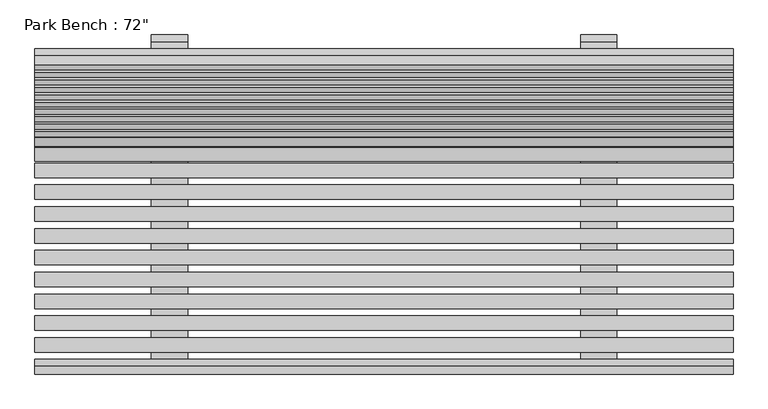
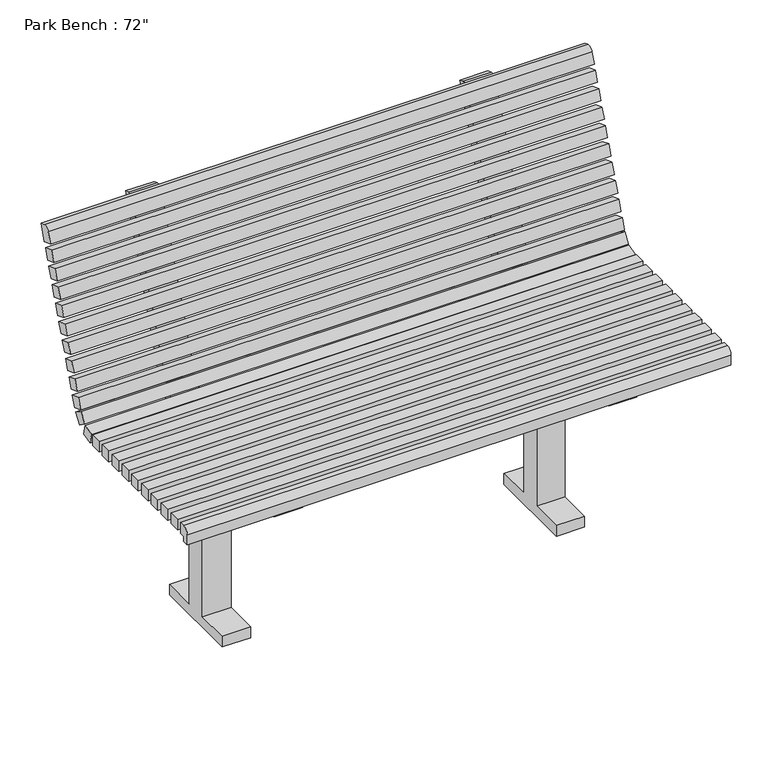
"""IFC4 building model written with IfcOpenShell, lengths in millimetres: geographic element geometry."""

from ifc_helpers import new_model, si_unit, point, frame, frame_2d, origin, place, context, project, spatial, polyline, circle_curve, trimmed, segment, composite_curve, outline, extrude, source, transform, mapped, element, save


def geographic_element_d8b57e58(model_context):
    return source(origin(), model_context, "Body", "SweptSolid", [
        extrude(outline(polyline([(609.6, -255.4337104), (609.6, -280.8337104), (-609.6, -280.8337104), (-609.6, -255.4337104), (609.6, -255.4337104)])), frame((0.0, 0.0, 457.2), z_axis=(0.0, 0.0, 1.0), x_axis=(1.0, 0.0, 0.0)), (0.0, 0.0, 1.0), 25.4),
        extrude(outline(polyline([(609.6, -217.3337104), (609.6, -242.7337104), (-609.6, -242.7337104), (-609.6, -217.3337104), (609.6, -217.3337104)])), frame((0.0, 0.0, 457.2), z_axis=(0.0, 0.0, 1.0), x_axis=(1.0, 0.0, 0.0)), (0.0, 0.0, 1.0), 25.4),
        extrude(outline(polyline([(609.6, -179.2337104), (609.6, -204.6337104), (-609.6, -204.6337104), (-609.6, -179.2337104), (609.6, -179.2337104)])), frame((0.0, 0.0, 457.2), z_axis=(0.0, 0.0, 1.0), x_axis=(1.0, 0.0, 0.0)), (0.0, 0.0, 1.0), 25.4),
        extrude(outline(polyline([(609.6, -141.1337104), (609.6, -166.5337104), (-609.6, -166.5337104), (-609.6, -141.1337104), (609.6, -141.1337104)])), frame((0.0, 0.0, 457.2), z_axis=(0.0, 0.0, 1.0), x_axis=(1.0, 0.0, 0.0)), (0.0, 0.0, 1.0), 25.4),
        extrude(outline(polyline([(609.6, -103.0337104), (609.6, -128.4337104), (-609.6, -128.4337104), (-609.6, -103.0337104), (609.6, -103.0337104)])), frame((0.0, 0.0, 457.2), z_axis=(0.0, 0.0, 1.0), x_axis=(1.0, 0.0, 0.0)), (0.0, 0.0, 1.0), 25.4),
        extrude(outline(polyline([(609.6, -64.9337104), (609.6, -90.3337104), (-609.6, -90.3337104), (-609.6, -64.9337104), (609.6, -64.9337104)])), frame((0.0, 0.0, 457.2), z_axis=(0.0, 0.0, 1.0), x_axis=(1.0, 0.0, 0.0)), (0.0, 0.0, 1.0), 25.4),
        extrude(outline(polyline([(609.6, -26.8337104), (609.6, -52.2337104), (-609.6, -52.2337104), (-609.6, -26.8337104), (609.6, -26.8337104)])), frame((0.0, 0.0, 457.2), z_axis=(0.0, 0.0, 1.0), x_axis=(1.0, 0.0, 0.0)), (0.0, 0.0, 1.0), 25.4),
        extrude(outline(polyline([(609.6, 11.2662896), (609.6, -14.1337104), (-609.6, -14.1337104), (-609.6, 11.2662896), (609.6, 11.2662896)])), frame((0.0, 0.0, 457.2), z_axis=(0.0, 0.0, 1.0), x_axis=(1.0, 0.0, 0.0)), (0.0, 0.0, 1.0), 25.4),
        extrude(outline(polyline([(609.6, 49.3662896), (609.6, 23.9662896), (-609.6, 23.9662896), (-609.6, 49.3662896), (609.6, 49.3662896)])), frame((0.0, 0.0, 457.2), z_axis=(0.0, 0.0, 1.0), x_axis=(1.0, 0.0, 0.0)), (0.0, 0.0, 1.0), 25.4),
        extrude(outline(composite_curve([segment(polyline([(-304.8, 457.2), (-304.8, 444.5), (-318.9337104, 444.5), (-318.9337104, 468.3125)]), True, "CONTINUOUS"), segment(trimmed(circle_curve(frame_2d((-304.6462104, 468.3125)), 14.2875), [point((-318.9337104, 468.3125))], [point((-304.6462104, 482.6))], False, "CARTESIAN"), True, "CONTINUOUS"), segment(polyline([(-304.6462104, 482.6), (-293.5337104, 482.6), (-293.5337104, 457.2), (-304.8, 457.2)]), True, "CONTINUOUS")], self_intersect=False)), frame((-609.6, 0.0, 0.0), z_axis=(1.0, 0.0, 0.0), x_axis=(0.0, 1.0, 0.0)), (0.0, 0.0, 1.0), 1219.2),
        extrude(outline(polyline([(0.0, -25.4), (0.0, 0.0), (1219.2, 0.0), (1219.2, -25.4), (0.0, -25.4)])), frame((609.6, 121.2738625, 585.5181247), z_axis=(0.0, 0.342020143325687, 0.9396926207859018), x_axis=(-1.0, 0.0, 0.0)), (0.0, 0.0, 1.0), 25.4),
        extrude(outline(polyline([(0.0, -25.4), (0.0, 0.0), (1219.2, 0.0), (1219.2, -25.4), (0.0, -25.4)])), frame((609.6, 134.30483, 621.3204136), z_axis=(0.0, 0.34202014332568254, 0.9396926207859034), x_axis=(-1.0, 0.0, 0.0)), (0.0, 0.0, 1.0), 25.4),
        extrude(outline(polyline([(0.0, -25.3999999), (0.0, 0.0), (1219.2, 0.0), (1219.2, -25.3999999), (0.0, -25.3999999)])), frame((609.6, 95.2119276, 513.913547), z_axis=(0.0, 0.34202014332568254, 0.9396926207859034), x_axis=(-1.0, 0.0, 0.0)), (0.0, 0.0, 1.0), 25.4),
        extrude(outline(polyline([(0.0, -25.4000001), (0.0, 0.0), (1219.2, 0.0), (1219.2, -25.4000001), (0.0, -25.4000001)])), frame((609.6, 108.242895, 549.7158359), z_axis=(0.0, 0.34202014332567804, 0.9396926207859051), x_axis=(-1.0, 0.0, 0.0)), (0.0, 0.0, 1.0), 25.4),
        extrude(outline(polyline([(0.0, -25.4), (0.0, 0.0), (1219.2, 0.0), (1219.2, -25.4), (0.0, -25.4)])), frame((609.6, 173.3977323, 728.7272801), z_axis=(0.0, 0.34202014332568337, 0.9396926207859031), x_axis=(-1.0, 0.0, 0.0)), (0.0, 0.0, 1.0), 25.4),
        extrude(outline(polyline([(0.0, -25.4000001), (0.0, 0.0), (1219.2, 0.0), (1219.2, -25.4000001), (0.0, -25.4000001)])), frame((609.6, 186.4286998, 764.529569), z_axis=(0.0, 0.3420201433256829, 0.9396926207859032), x_axis=(-1.0, 0.0, 0.0)), (0.0, 0.0, 1.0), 25.4),
        extrude(outline(polyline([(0.0, -25.4), (0.0, 0.0), (1219.2, 0.0), (1219.2, -25.4), (0.0, -25.4)])), frame((609.6, 147.3357974, 657.1227024), z_axis=(0.0, 0.3420201433256776, 0.9396926207859052), x_axis=(-1.0, 0.0, 0.0)), (0.0, 0.0, 1.0), 25.4),
        extrude(outline(polyline([(0.0, -25.4), (0.0, 0.0), (1219.2, 0.0), (1219.2, -25.4), (0.0, -25.4)])), frame((609.6, 160.3667649, 692.9249913), z_axis=(0.0, 0.34202014332568254, 0.9396926207859034), x_axis=(-1.0, 0.0, 0.0)), (0.0, 0.0, 1.0), 25.4),
        extrude(outline(polyline([(0.0, -25.3999999), (0.0, 0.0), (1219.2, 0.0), (1219.2, -25.3999999), (0.0, -25.3999999)])), frame((609.6, 199.4596673, 800.3318578), z_axis=(0.0, 0.3420201433256774, 0.9396926207859052), x_axis=(-1.0, 0.0, 0.0)), (0.0, 0.0, 1.0), 25.4),
        extrude(outline(composite_curve([segment(polyline([(249.3897948, 863.2491239), (236.3588273, 827.4468351), (212.4906347, 836.1341467), (221.1779464, 860.0023393)]), True, "CONTINUOUS"), segment(trimmed(circle_curve(frame_2d((233.1120426, 855.6586834)), 12.7), [point((221.1779464, 860.0023393))], [point((237.4556985, 867.5927797))], False, "CARTESIAN"), True, "CONTINUOUS"), segment(polyline([(237.4556985, 867.5927797), (249.3897948, 863.2491239)]), True, "CONTINUOUS")], self_intersect=False)), frame((-609.6, 0.0, 0.0), z_axis=(1.0, 0.0, 0.0), x_axis=(0.0, 1.0, 0.0)), (0.0, 0.0, 1.0), 1219.2),
        extrude(outline(polyline([(0.0, -25.4), (0.0, 0.0), (1219.2, 0.0), (1219.2, -25.4), (0.0, -25.4)])), frame((609.6, 78.7855779, 490.7267336), z_axis=(0.0, 0.5735764363510742, 0.8191520442889721), x_axis=(-1.0, 0.0, 0.0)), (0.0, 0.0, 1.0), 25.4),
        extrude(outline(polyline([(0.0, -25.4), (0.0, 0.0), (1219.2, 0.0), (1219.2, -25.4), (0.0, -25.4)])), frame((609.6, 59.0817015, 457.2297909), z_axis=(0.0, -0.2588190451024684, 0.9659258262890824), x_axis=(-1.0, 0.0, 0.0)), (0.0, 0.0, 1.0), 25.4),
        extrude(outline(composite_curve([segment(polyline([(-101.6, 25.4), (-25.4, 25.4), (-25.4, 431.8), (-304.8, 431.8), (-304.8, 457.2), (57.1368213, 457.2)]), True, "CONTINUOUS"), segment(trimmed(circle_curve(frame_2d((57.1368213, 520.7)), 63.5), [point((57.1368213, 457.2))], [point((116.8073027, 498.9817209))], True, "CARTESIAN"), True, "CONTINUOUS"), segment(polyline([(116.8073027, 498.9817209), (244.9406421, 851.0251774)]), True, "CONTINUOUS"), segment(trimmed(circle_curve(frame_2d((256.8747384, 846.6815216)), 12.7), [point((244.9406421, 851.0251774))], [point((261.2183942, 858.6156178))], False, "CARTESIAN"), True, "CONTINUOUS"), segment(polyline([(261.2183942, 858.6156178), (273.1524905, 854.271962), (140.6754953, 490.2944093)]), True, "CONTINUOUS"), segment(trimmed(circle_curve(frame_2d((57.1368213, 520.7)), 88.9), [point((140.6754953, 490.2944093))], [point((57.1368213, 431.8))], False, "CARTESIAN"), True, "CONTINUOUS"), segment(polyline([(57.1368213, 431.8), (25.4, 431.8), (25.4, 25.4), (101.6, 25.4), (101.6, 0.0), (-101.6, 0.0), (-101.6, 25.4)]), True, "CONTINUOUS")], self_intersect=False)), frame((343.5736591, 0.0, 0.0), z_axis=(1.0, 0.0, 0.0), x_axis=(0.0, 1.0, 0.0)), (0.0, 0.0, 1.0), 62.8263409),
        extrude(outline(composite_curve([segment(polyline([(-101.6, 25.4), (-25.4, 25.4), (-25.4, 431.8), (-304.8, 431.8), (-304.8, 457.2), (57.1368213, 457.2)]), True, "CONTINUOUS"), segment(trimmed(circle_curve(frame_2d((57.1368213, 520.7)), 63.5), [point((57.1368213, 457.2))], [point((116.8073027, 498.9817209))], True, "CARTESIAN"), True, "CONTINUOUS"), segment(polyline([(116.8073027, 498.9817209), (244.9406421, 851.0251774)]), True, "CONTINUOUS"), segment(trimmed(circle_curve(frame_2d((256.8747384, 846.6815216)), 12.7), [point((244.9406421, 851.0251774))], [point((261.2183942, 858.6156178))], False, "CARTESIAN"), True, "CONTINUOUS"), segment(polyline([(261.2183942, 858.6156178), (273.1524905, 854.271962), (140.6754953, 490.2944093)]), True, "CONTINUOUS"), segment(trimmed(circle_curve(frame_2d((57.1368213, 520.7)), 88.9), [point((140.6754953, 490.2944093))], [point((57.1368213, 431.8))], False, "CARTESIAN"), True, "CONTINUOUS"), segment(polyline([(57.1368213, 431.8), (25.4, 431.8), (25.4, 25.4), (101.6, 25.4), (101.6, 0.0), (-101.6, 0.0), (-101.6, 25.4)]), True, "CONTINUOUS")], self_intersect=False)), frame((-406.4, 0.0, 0.0), z_axis=(1.0, 0.0, 0.0), x_axis=(0.0, 1.0, 0.0)), (0.0, 0.0, 1.0), 63.8916859),
    ])


if __name__ == "__main__":
    model = new_model("IFC4")
    model_context = context("Model", 3, world=origin())
    ifc_project = project(units=[si_unit("LENGTHUNIT", "METRE", prefix="MILLI")], contexts=[model_context])
    site = spatial("IfcSite", under=ifc_project)
    building = spatial("IfcBuilding", under=site)
    placement = place(None, origin())
    geographic_element_shape = geographic_element_d8b57e58(model_context)
    element("IfcGeographicElement", 1, ObjectType="Park Bench : 72\"", at=placement, inside=building, context=model_context, shape_type="MappedRepresentation", body=[
        mapped(geographic_element_shape, transform((0.0, 0.0, 0.0), x_axis=(1.0, 0.0, 0.0), y_axis=(0.0, 1.0, 0.0), z_axis=(0.0, 0.0, 1.0))),
    ])
    save(model, "model.ifc")

# Revit data of these elements
# Type "Park Bench : 72\""
#   Length = 4' - 0"
#   Seat Material = Wood - Teak
#   Frame Material = Steel, Paint Finish, Dark Gray, Matte
# Element 1 (IfcGeographicElement, "Park Bench : 72\"")
#   Materials on its faces: "Wood - Teak", "Steel, Paint Finish, Dark Gray, Matte"
# Materials
#   "Wood - Teak": class "Wood", colour RGB 120 73 19, transparency 0
#   "Steel, Paint Finish, Dark Gray, Matte": class "Metal", colour RGB 98 98 98, transparency 0, Description = "Steel, paint finish, dark gray, matte", Cost = 0
